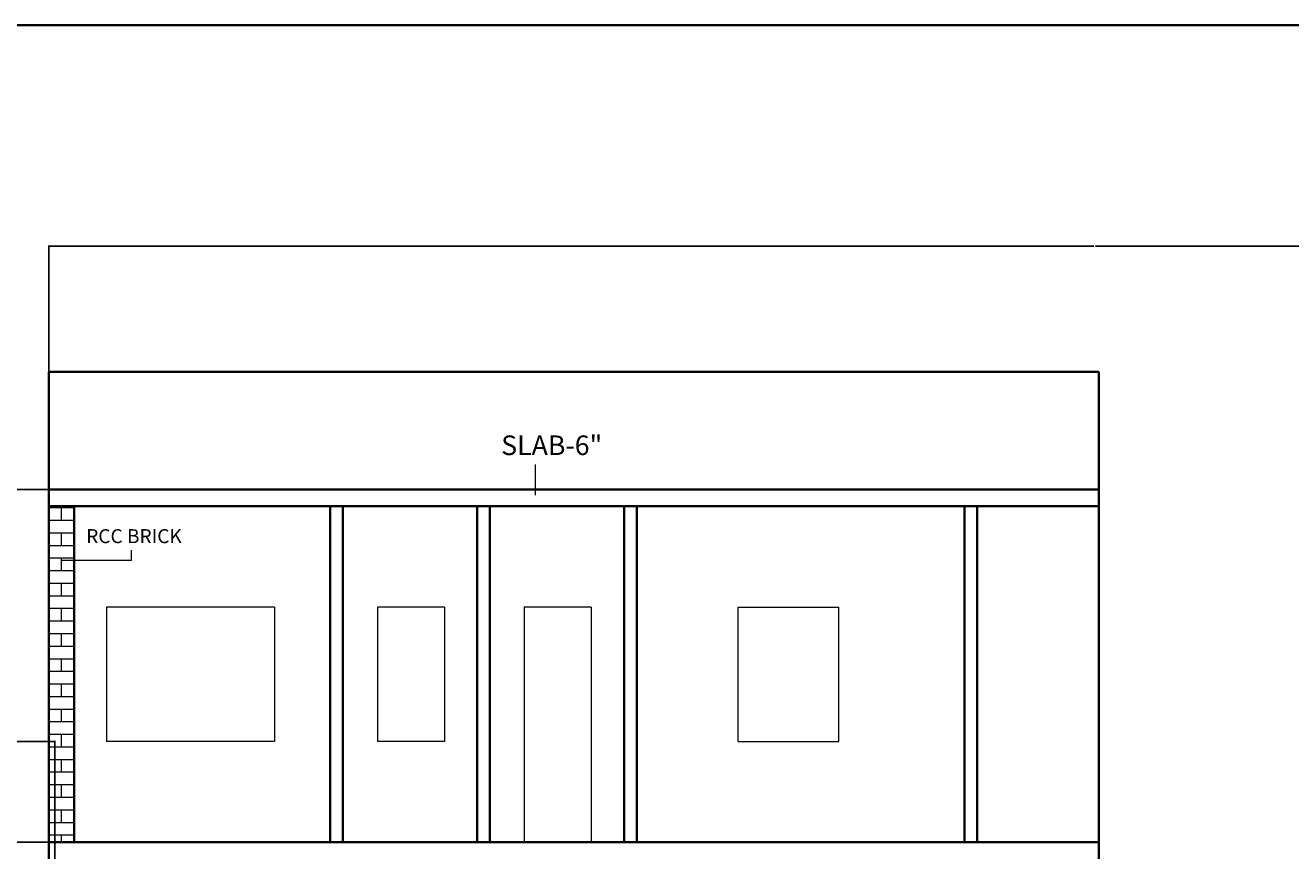
# Model space of a CAD drawing. Units: inches. Extents: x 2120 to 4013, y 1390 to 3019.
# Tile 58 of 59: x 3063 to 3515, y 2724 to 3019. Entities that reach past the tile are written whole.
import ezdxf

# ---------------------------------------------------------------- set-up
doc = ezdxf.new("R2010")
doc.units = ezdxf.units.IN
for name, color, linetype, lineweight in [('A-ANNO-DIMS', 2, 'Continuous', 18), ('A-ANNO-TEXT', 7, 'Continuous', 18), ('A-ANNO-TTLB', 7, 'Continuous', 35), ('A-DOOR', 3, 'Continuous', 18), ('A-GLAZ', 4, 'Continuous', 18), ('A-SECT', 7, 'Continuous', 35), ('A-WALL-PATT', 252, 'Continuous', 13)]:
    doc.layers.add(name, color=color, linetype=linetype, lineweight=lineweight)
doc.styles.get("Standard").update_dxf_attribs({"font": 'arial.ttf'})
doc.dimstyles.get("Standard").update_dxf_attribs({"dimtxt": 0.18, "dimasz": 0.18, "dimexe": 0.18, "dimexo": 0.0625, "dimgap": 0.09, "dimtad": 0, "dimtih": 1, "dimtoh": 1, "dimdec": 4, "dimzin": 0, "dimdsep": 46, "dimtxsty": 'Standard', "dimcen": 0.09, "dimadec": 0, "dimazin": 0, "dimtfac": 1, "dimtdec": 4, "dimtofl": 0, "dimtmove": 0, "dimatfit": 3, "dimfxl": 1, "dimtolj": 1, "dimtzin": 0, "dimarcsym": 0})

# ---------------------------------------------------------------- blocks, each defined once
blk = doc.blocks.new('WIN-SECT-60IN')
for p, q in [((0, 48), (0, 0)), ((60, 48), (0, 48)), ((60, 48), (60, 0)), ((60, 0), (0, 0))]:
    blk.add_line(p, q)
blk = doc.blocks.new('WIN-SECT-24IN')
for p, q in [((0, 48), (0, 0)), ((0, 48), (0, 0)), ((24, 48), (0, 48)), ((24, 48), (24, 0)), ((24, 0), (0, 0))]:
    blk.add_line(p, q)
blk = doc.blocks.new('DOOR-SECT-24IN')
for p, q in [((0, 84), (0, 0)), ((24, 84), (0, 84)), ((24, 84), (24, 0))]:
    blk.add_line(p, q)
blk = doc.blocks.new('WIN-SECT-36IN')
for p, q in [((0, 48), (0, 0)), ((36, 48), (0, 48)), ((36, 48), (36, 0)), ((36, 0), (0, 0))]:
    blk.add_line(p, q)
blk = doc.blocks.new('*D235')
at = {"layer": 'A-ANNO-DIMS', "color": 0, "lineweight": -2, "transparency": 16777216}
for p, q in [((3033.8, 2763.31), (3074.11, 2763.31)), ((3073.93, 2763.13), (3073.93, 2703.49)), ((3073.93, 2643.49), (3073.93, 2703.13)), ((3033.8, 2643.31), (3074.11, 2643.31))]:
    blk.add_line(p, q, dxfattribs=at)
at = {"layer": 'A-ANNO-DIMS', "color": 0, "transparency": 16777216}
for points in [[(3073.9, 2763.13), (3073.96, 2763.13), (3073.93, 2763.31)], [(3073.9, 2643.49), (3073.96, 2643.49), (3073.93, 2643.31)]]:
    blk.add_solid(points, dxfattribs=at)
at = {"layer": 'Defpoints', "color": 0, "transparency": 16777216}
for p in [(3033.73, 2763.31), (3073.93, 2763.31), (3033.73, 2643.31)]:
    blk.add_point(p, dxfattribs=at)
at = {"layer": 'A-ANNO-DIMS', "color": 0, "transparency": 16777216, "insert": (3073.93, 2703.31), "char_height": 0.18, "attachment_point": 5}
blk.add_mtext('\\A1;120', dxfattribs=at)
blk = doc.blocks.new('*D236')
at = {"layer": 'A-ANNO-DIMS', "color": 0, "lineweight": -2, "transparency": 16777216}
for p, q in [((3071.73, 2895.37), (3071.73, 2940.44)), ((3071.91, 2940.26), (3444.95, 2940.26)), ((3818.55, 2940.26), (3445.52, 2940.26)), ((3818.73, 2895.37), (3818.73, 2940.44))]:
    blk.add_line(p, q, dxfattribs=at)
at = {"layer": 'A-ANNO-DIMS', "color": 0, "transparency": 16777216}
for points in [[(3071.91, 2940.29), (3071.91, 2940.23), (3071.73, 2940.26)], [(3818.55, 2940.29), (3818.55, 2940.23), (3818.73, 2940.26)]]:
    blk.add_solid(points, dxfattribs=at)
at = {"layer": 'Defpoints', "color": 0, "transparency": 16777216}
for p in [(3818.73, 2940.26), (3071.73, 2895.31), (3818.73, 2895.31)]:
    blk.add_point(p, dxfattribs=at)
at = {"layer": 'A-ANNO-DIMS', "color": 0, "transparency": 16777216, "insert": (3445.23, 2940.26), "char_height": 0.18, "attachment_point": 5}
blk.add_mtext('\\A1;747', dxfattribs=at)
blk = doc.blocks.new('*D239')
at = {"layer": 'A-ANNO-DIMS', "color": 0, "lineweight": -2, "transparency": 16777216}
for p, q in [((3071.67, 2727.31), (3026.6, 2727.31)), ((3026.78, 2727.13), (3026.78, 2664.49)), ((3026.78, 2601.49), (3026.78, 2664.13)), ((3071.67, 2601.31), (3026.6, 2601.31))]:
    blk.add_line(p, q, dxfattribs=at)
at = {"layer": 'A-ANNO-DIMS', "color": 0, "transparency": 16777216}
for points in [[(3026.75, 2727.13), (3026.81, 2727.13), (3026.78, 2727.31)], [(3026.75, 2601.49), (3026.81, 2601.49), (3026.78, 2601.31)]]:
    blk.add_solid(points, dxfattribs=at)
at = {"layer": 'Defpoints', "color": 0, "transparency": 16777216}
for p in [(3026.78, 2727.31), (3071.73, 2727.31), (3071.73, 2601.31)]:
    blk.add_point(p, dxfattribs=at)
at = {"layer": 'A-ANNO-DIMS', "color": 0, "transparency": 16777216, "insert": (3026.78, 2664.31), "char_height": 0.18, "attachment_point": 5}
blk.add_mtext('\\A1;126', dxfattribs=at)
blk = doc.blocks.new('*D240')
at = {"layer": 'A-ANNO-DIMS', "color": 0, "lineweight": -2, "transparency": 16777216}
for p, q in [((3071.67, 2853.31), (3026.6, 2853.31)), ((3026.78, 2853.13), (3026.78, 2790.49)), ((3026.78, 2727.49), (3026.78, 2790.13)), ((3071.67, 2727.31), (3026.6, 2727.31))]:
    blk.add_line(p, q, dxfattribs=at)
at = {"layer": 'A-ANNO-DIMS', "color": 0, "transparency": 16777216}
for points in [[(3026.75, 2853.13), (3026.81, 2853.13), (3026.78, 2853.31)], [(3026.75, 2727.49), (3026.81, 2727.49), (3026.78, 2727.31)]]:
    blk.add_solid(points, dxfattribs=at)
at = {"layer": 'Defpoints', "color": 0, "transparency": 16777216}
for p in [(3026.78, 2853.31), (3071.73, 2853.31), (3071.73, 2727.31)]:
    blk.add_point(p, dxfattribs=at)
at = {"layer": 'A-ANNO-DIMS', "color": 0, "transparency": 16777216, "insert": (3026.78, 2790.31), "char_height": 0.18, "attachment_point": 5}
blk.add_mtext('\\A1;126', dxfattribs=at)

msp = doc.modelspace()

# ---------------------------------------------------------------- hatches: boundary and pattern name
at = {"layer": 'A-WALL-PATT'}
h = msp.add_hatch(dxfattribs=at)
h.set_pattern_fill('BRICK', color=256, scale=0.708254, style=0)
h.paths.add_polyline_path([(3071.7347, 2727.3118), (3080.7347, 2727.3118), (3080.7347, 2847.3118), (3071.7347, 2847.3118)])

# ---------------------------------------------------------------- linework, layer by layer
at = {"layer": 'A-ANNO-TEXT'}
for p, q in [((3245.5564, 2851.3475), (3245.5564, 2862.2403)), ((3101.3172, 2828.1101), (3101.3172, 2831.6769)), ((3076.2347, 2828.1101), (3101.3172, 2828.1101))]:
    msp.add_line(p, q, dxfattribs=at)
at = {"layer": 'A-ANNO-TTLB'}
msp.add_lwpolyline([(2120.4581, 3019.1237), (4012.9334, 3019.1237), (4012.9334, 1390.2222), (2120.4581, 1390.2222)], close=True, dxfattribs=at)
at = {"layer": 'A-SECT'}
for p, q in [((3071.7347, 2895.3118), (3071.7347, 2709.3118)), ((3446.7347, 2895.3118), (3071.7347, 2895.3118)), ((3446.7347, 2895.3118), (3446.7347, 2727.3118)), ((3446.7347, 2853.3118), (3071.7347, 2853.3118)), ((3446.7347, 2847.3118), (3071.7347, 2847.3118)), ((3080.7347, 2847.3118), (3080.7347, 2727.3118)), ((3172.2347, 2847.3118), (3172.2347, 2727.3118)), ((3176.7347, 2847.3118), (3176.7347, 2727.3118)), ((3224.7347, 2847.3118), (3224.7347, 2727.3118)), ((3224.7347, 2847.3118), (3224.7347, 2727.3118)), ((3229.2347, 2847.3118), (3229.2347, 2727.3118)), ((3277.2347, 2847.3118), (3277.2347, 2727.3118)), ((3281.7347, 2847.3118), (3281.7347, 2727.3118)), ((3398.7347, 2847.3118), (3398.7347, 2727.3118)), ((3403.2347, 2847.3118), (3403.2347, 2727.3118)), ((3071.7347, 2769.3118), (3071.7347, 2583.3118)), ((3446.7347, 2727.3118), (3071.7347, 2727.3118)), ((3446.7347, 2727.3118), (3446.7347, 2595.3118))]:
    msp.add_line(p, q, dxfattribs=at)

# ---------------------------------------------------------------- block references
at = {"layer": 'A-DOOR'}
msp.add_blockref('DOOR-SECT-24IN', (3241.4354, 2727.3118), dxfattribs=at)
at = {"layer": 'A-GLAZ'}
for name, p in [('WIN-SECT-60IN', (3092.3803, 2763.3118)), ('WIN-SECT-24IN', (3189.0958, 2763.3118))]:
    msp.add_blockref(name, p, dxfattribs=at)
at = {"layer": 'A-GLAZ', "rotation": 180}
msp.add_blockref('WIN-SECT-36IN', (3353.9131, 2811.3118), dxfattribs=at)

# ---------------------------------------------------------------- texts
at = {"layer": 'A-ANNO-TEXT', "attachment_point": 1}
for s, width, insert, char_height in [('SLAB-6"', 93.254406, (3233.2765, 2872.6238), 7), ('RCC BRICK', 48.947981, (3085.0697, 2839.1594), 5)]:
    msp.add_mtext_dynamic_manual_height_columns(s, width=width, gutter_width=12.5, heights=[0], dxfattribs=dict(at, insert=insert, char_height=char_height))

# ---------------------------------------------------------------- dimensions: what is measured, and where the dimension line sits
at = {"layer": 'A-ANNO-DIMS'}
dim = msp.add_linear_dim(base=(3818.7347, 2940.2618), p1=(3071.7347, 2895.3118), p2=(3818.7347, 2895.3118), dimstyle='Standard', override={"dimdec": 0, "dimlfac": 1, "dimrnd": 0, "dimzin": 0, "dimdsep": 46, "dimlunit": 2}, dxfattribs=at)
dim.commit()
dim.dimension.update_dxf_attribs({"geometry": '*D236', "text_midpoint": (3445.2347, 2940.2618)})
for base, p1, p2, picture, middle in [((3026.7847, 2853.3118), (3071.7347, 2727.3118), (3071.7347, 2853.3118), '*D240', (3026.7847, 2790.3118)), ((3073.9331, 2763.3118), (3033.7331, 2643.3118), (3033.7331, 2763.3118), '*D235', (3073.9331, 2703.3118)), ((3026.7847, 2727.3118), (3071.7347, 2601.3118), (3071.7347, 2727.3118), '*D239', (3026.7847, 2664.3118))]:
    dim = msp.add_linear_dim(base=base, p1=p1, p2=p2, angle=90, dimstyle='Standard', override={"dimdec": 0, "dimlfac": 1, "dimrnd": 0, "dimzin": 0, "dimdsep": 46, "dimlunit": 2}, dxfattribs=at)
    dim.commit()
    dim.dimension.update_dxf_attribs({"geometry": picture, "text_midpoint": middle})

doc.saveas('drawing.dxf')
